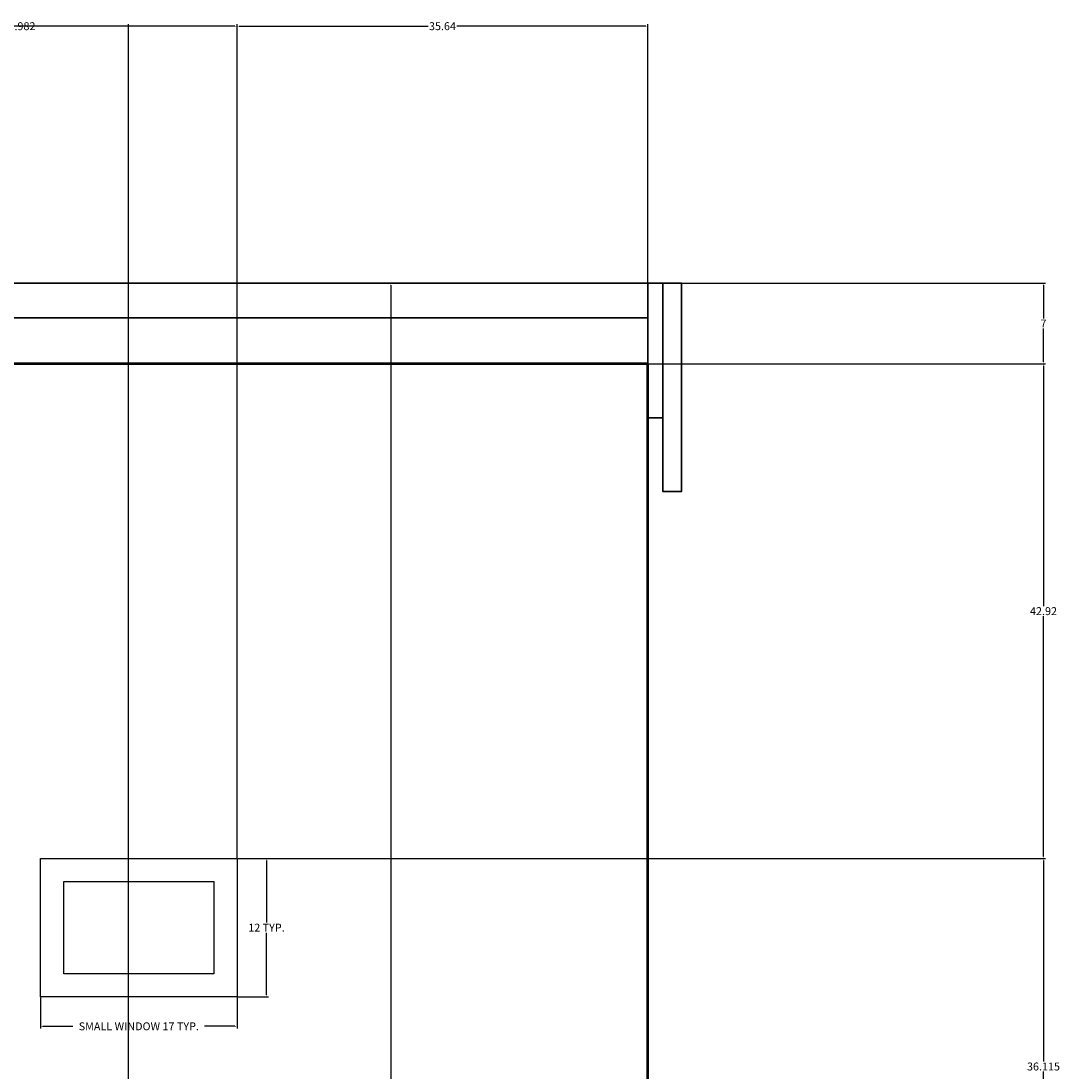
# Model space of a CAD drawing. Units: inches. Extents: x -139 to 346, y 72 to 413.
# Tile 18 of 18: x 256 to 346, y 322 to 413. Entities that reach past the tile are written whole.
import ezdxf

# ---------------------------------------------------------------- set-up
doc = ezdxf.new("R2010")
doc.units = ezdxf.units.IN
doc.header["$MEASUREMENT"] = 0
for name, color, linetype, lineweight in [('A-ANNO-DIMS', 2, 'Continuous', 18), ('A-GLAZ', 4, 'Continuous', 25), ('A-ROOF', 1, 'Continuous', 35), ('A-WALL', 7, 'Continuous', 50)]:
    doc.layers.add(name, color=color, linetype=linetype, lineweight=lineweight)
doc.styles.get("Standard").update_dxf_attribs({"font": 'arial.ttf'})
doc.dimstyles.get("Standard").update_dxf_attribs({"dimtxt": 0.6875, "dimasz": 0.18, "dimexe": 0.18, "dimexo": 0.0625, "dimgap": 0.09, "dimtad": 0, "dimtih": 1, "dimtoh": 1, "dimdec": 4, "dimzin": 0, "dimdsep": 46, "dimlunit": 4, "dimtxsty": 'Standard', "dimcen": 0.09, "dimadec": 0, "dimazin": 0, "dimtfac": 1, "dimtdec": 4, "dimtofl": 0, "dimtmove": 0, "dimatfit": 3, "dimfxl": 1, "dimtolj": 1, "dimtzin": 0, "dimarcsym": 0})

# ---------------------------------------------------------------- blocks, each defined once
blk = doc.blocks.new('WIN-SMALL')
for points in [[(0, 12.015), (17.035, 12.015), (17.035, 0), (0, 0)], [(2, 10.015), (15.035, 10.015), (15.035, 2), (2, 2)]]:
    blk.add_lwpolyline(points, close=True)
blk = doc.blocks.new('*D5')
at = {"layer": 'A-ANNO-DIMS', "color": 0, "lineweight": -2, "transparency": 16777216}
for p, q in [((257.212, 327.977), (257.212, 325.305)), ((274.247, 327.977), (274.247, 325.305)), ((257.392, 325.485), (260.019, 325.485)), ((274.067, 325.485), (271.439, 325.485))]:
    blk.add_line(p, q, dxfattribs=at)
at = {"layer": 'A-ANNO-DIMS', "color": 0, "transparency": 16777216}
for points in [[(257.392, 325.515), (257.392, 325.455), (257.212, 325.485)], [(274.067, 325.515), (274.067, 325.455), (274.247, 325.485)]]:
    blk.add_solid(points, dxfattribs=at)
at = {"layer": 'Defpoints', "color": 0, "transparency": 16777216}
for p in [(257.212, 328.04), (274.247, 328.04), (274.247, 325.485)]:
    blk.add_point(p, dxfattribs=at)
at = {"layer": 'A-ANNO-DIMS', "color": 0, "transparency": 16777216, "insert": (265.729, 325.485), "char_height": 0.6875, "attachment_point": 5}
blk.add_mtext('\\A1;SMALL WINDOW 17 TYP.', dxfattribs=at)
blk = doc.blocks.new('*D6')
at = {"layer": 'A-ANNO-DIMS', "color": 0, "lineweight": -2, "transparency": 16777216}
for p, q in [((274.309, 340.055), (276.982, 340.055)), ((276.802, 339.875), (276.802, 334.483)), ((276.802, 328.22), (276.802, 333.612)), ((274.309, 328.04), (276.982, 328.04))]:
    blk.add_line(p, q, dxfattribs=at)
at = {"layer": 'A-ANNO-DIMS', "color": 0, "transparency": 16777216}
for points in [[(276.772, 339.875), (276.832, 339.875), (276.802, 340.055)], [(276.772, 328.22), (276.832, 328.22), (276.802, 328.04)]]:
    blk.add_solid(points, dxfattribs=at)
at = {"layer": 'Defpoints', "color": 0, "transparency": 16777216}
for p in [(274.247, 340.055), (276.802, 340.055), (274.247, 328.04)]:
    blk.add_point(p, dxfattribs=at)
at = {"layer": 'A-ANNO-DIMS', "color": 0, "transparency": 16777216, "insert": (276.802, 334.047), "char_height": 0.6875, "attachment_point": 5}
blk.add_mtext('\\A1;12 TYP.', dxfattribs=at)
blk = doc.blocks.new('*D28')
at = {"layer": 'A-ANNO-DIMS', "color": 0, "lineweight": -2, "transparency": 16777216}
for p, q in [((175.668, 340.117), (175.668, 412.455)), ((175.848, 412.275), (223.706, 412.275)), ((274.067, 412.275), (226.208, 412.275)), ((274.247, 340.117), (274.247, 412.455))]:
    blk.add_line(p, q, dxfattribs=at)
at = {"layer": 'A-ANNO-DIMS', "color": 0, "transparency": 16777216}
for points in [[(175.848, 412.305), (175.848, 412.245), (175.668, 412.275)], [(274.067, 412.305), (274.067, 412.245), (274.247, 412.275)]]:
    blk.add_solid(points, dxfattribs=at)
at = {"layer": 'Defpoints', "color": 0, "transparency": 16777216}
for p in [(274.247, 412.275), (175.668, 340.055), (274.247, 340.055)]:
    blk.add_point(p, dxfattribs=at)
at = {"layer": 'A-ANNO-DIMS', "color": 0, "transparency": 16777216, "insert": (224.957, 412.275), "char_height": 0.6875, "attachment_point": 5}
blk.add_mtext('\\A1;98.58', dxfattribs=at)
blk = doc.blocks.new('*D29')
at = {"layer": 'A-ANNO-DIMS', "color": 0, "lineweight": -2, "transparency": 16777216}
for p, q in [((274.247, 340.117), (274.247, 412.455)), ((274.427, 412.275), (290.82, 412.275)), ((309.709, 412.275), (293.316, 412.275)), ((309.889, 383.037), (309.889, 412.455))]:
    blk.add_line(p, q, dxfattribs=at)
at = {"layer": 'A-ANNO-DIMS', "color": 0, "transparency": 16777216}
for points in [[(274.427, 412.305), (274.427, 412.245), (274.247, 412.275)], [(309.709, 412.305), (309.709, 412.245), (309.889, 412.275)]]:
    blk.add_solid(points, dxfattribs=at)
at = {"layer": 'Defpoints', "color": 0, "transparency": 16777216}
for p in [(309.889, 412.275), (309.889, 382.975), (274.247, 340.055)]:
    blk.add_point(p, dxfattribs=at)
at = {"layer": 'A-ANNO-DIMS', "color": 0, "transparency": 16777216, "insert": (292.068, 412.275), "char_height": 0.6875, "attachment_point": 5}
blk.add_mtext('\\A1;35.64', dxfattribs=at)
blk = doc.blocks.new('*D31')
at = {"layer": 'A-ANNO-DIMS', "color": 0, "lineweight": -2, "transparency": 16777216}
for p, q in [((309.827, 389.975), (287.409, 389.975)), ((287.589, 389.795), (287.589, 242.916)), ((287.589, 95.155), (287.589, 242.034)), ((309.827, 94.975), (287.409, 94.975))]:
    blk.add_line(p, q, dxfattribs=at)
at = {"layer": 'A-ANNO-DIMS', "color": 0, "transparency": 16777216}
for points in [[(287.559, 389.795), (287.619, 389.795), (287.589, 389.975)], [(287.559, 95.155), (287.619, 95.155), (287.589, 94.975)]]:
    blk.add_solid(points, dxfattribs=at)
at = {"layer": 'Defpoints', "color": 0, "transparency": 16777216}
for p in [(287.589, 389.975), (309.889, 389.975), (309.889, 94.975)]:
    blk.add_point(p, dxfattribs=at)
at = {"layer": 'A-ANNO-DIMS', "color": 0, "transparency": 16777216, "insert": (287.589, 242.475), "char_height": 0.6875, "attachment_point": 5}
blk.add_mtext('\\A1;295', dxfattribs=at)
blk = doc.blocks.new('*D35')
at = {"layer": 'A-ANNO-DIMS', "color": 0, "lineweight": -2, "transparency": 16777216}
for p, q in [((274.309, 340.055), (344.386, 340.055)), ((344.206, 339.875), (344.206, 322.439)), ((344.206, 304.12), (344.206, 321.556)), ((274.309, 303.94), (344.386, 303.94))]:
    blk.add_line(p, q, dxfattribs=at)
at = {"layer": 'A-ANNO-DIMS', "color": 0, "transparency": 16777216}
for points in [[(344.176, 339.875), (344.236, 339.875), (344.206, 340.055)], [(344.176, 304.12), (344.236, 304.12), (344.206, 303.94)]]:
    blk.add_solid(points, dxfattribs=at)
at = {"layer": 'Defpoints', "color": 0, "transparency": 16777216}
for p in [(274.247, 340.055), (344.206, 340.055), (274.247, 303.94)]:
    blk.add_point(p, dxfattribs=at)
at = {"layer": 'A-ANNO-DIMS', "color": 0, "transparency": 16777216, "insert": (344.206, 321.998), "char_height": 0.6875, "attachment_point": 5}
blk.add_mtext('\\A1;36.115', dxfattribs=at)
blk = doc.blocks.new('*D36')
at = {"layer": 'A-ANNO-DIMS', "color": 0, "lineweight": -2, "transparency": 16777216}
for p, q in [((309.952, 382.975), (344.386, 382.975)), ((344.206, 382.795), (344.206, 361.956)), ((344.206, 340.235), (344.206, 361.074)), ((274.309, 340.055), (344.386, 340.055))]:
    blk.add_line(p, q, dxfattribs=at)
at = {"layer": 'A-ANNO-DIMS', "color": 0, "transparency": 16777216}
for points in [[(344.176, 382.795), (344.236, 382.795), (344.206, 382.975)], [(344.176, 340.235), (344.236, 340.235), (344.206, 340.055)]]:
    blk.add_solid(points, dxfattribs=at)
at = {"layer": 'Defpoints', "color": 0, "transparency": 16777216}
for p in [(309.889, 382.975), (344.206, 382.975), (274.247, 340.055)]:
    blk.add_point(p, dxfattribs=at)
at = {"layer": 'A-ANNO-DIMS', "color": 0, "transparency": 16777216, "insert": (344.206, 361.515), "char_height": 0.6875, "attachment_point": 5}
blk.add_mtext('\\A1;42.92', dxfattribs=at)
blk = doc.blocks.new('*D37')
at = {"layer": 'A-ANNO-DIMS', "color": 0, "lineweight": -2, "transparency": 16777216}
for p, q in [((309.951928, 389.974785), (344.385522, 389.974785)), ((344.205522, 389.794785), (344.205522, 386.908535)), ((344.205522, 383.154785), (344.205522, 386.041035)), ((309.951928, 382.974785), (344.385522, 382.974785))]:
    blk.add_line(p, q, dxfattribs=at)
at = {"layer": 'A-ANNO-DIMS', "color": 0, "transparency": 16777216}
for points in [[(344.175522, 389.794785), (344.235522, 389.794785), (344.205522, 389.974785)], [(344.175522, 383.154785), (344.235522, 383.154785), (344.205522, 382.974785)]]:
    blk.add_solid(points, dxfattribs=at)
at = {"layer": 'Defpoints', "color": 0, "transparency": 16777216}
for p in [(309.889428, 389.974785), (344.205522, 389.974785), (309.889428, 382.974785)]:
    blk.add_point(p, dxfattribs=at)
at = {"layer": 'A-ANNO-DIMS', "color": 0, "transparency": 16777216, "insert": (344.205522, 386.474785), "char_height": 0.6875, "attachment_point": 5}
blk.add_mtext('\\A1;7', dxfattribs=at)
blk = doc.blocks.new('*D82')
at = {"layer": 'A-ANNO-DIMS', "color": 0, "lineweight": -2, "transparency": 16777216}
for p, q in [((245.84, 184.668), (245.84, 412.455)), ((246.02, 412.275), (253.85, 412.275)), ((264.642, 412.275), (256.812, 412.275)), ((264.822, 184.668), (264.822, 412.455))]:
    blk.add_line(p, q, dxfattribs=at)
at = {"layer": 'A-ANNO-DIMS', "color": 0, "transparency": 16777216}
for points in [[(246.02, 412.305), (246.02, 412.245), (245.84, 412.275)], [(264.642, 412.305), (264.642, 412.245), (264.822, 412.275)]]:
    blk.add_solid(points, dxfattribs=at)
at = {"layer": 'Defpoints', "color": 0, "transparency": 16777216}
for p in [(264.822, 412.275), (245.84, 184.606), (264.822, 184.606)]:
    blk.add_point(p, dxfattribs=at)
at = {"layer": 'A-ANNO-DIMS', "color": 0, "transparency": 16777216, "insert": (255.331, 412.275), "char_height": 0.6875, "attachment_point": 5}
blk.add_mtext('\\A1;18.982', dxfattribs=at)

msp = doc.modelspace()

# ---------------------------------------------------------------- linework, layer by layer
at = {"layer": 'A-ROOF'}
for p, q in [((-47.2734, 389.9748), (309.8894, 389.9748)), ((309.8894, 389.9748), (309.8894, 386.9223)), ((-47.2734, 386.9748), (309.8894, 386.9748)), ((309.8894, 386.9748), (309.8894, 382.9748))]:
    msp.add_line(p, q, dxfattribs=at)
for points in [[(309.8894, 389.9748), (311.1776, 389.9748), (311.1776, 378.2896), (309.8894, 378.2896)], [(311.1776, 389.9748), (312.8172, 389.9748), (312.8172, 371.9089), (311.1776, 371.9089)]]:
    msp.add_lwpolyline(points, close=True, dxfattribs=at)
at = {"layer": 'A-WALL'}
for p, q in [((309.8894, 382.9748), (89.4597, 382.9748)), ((309.8894, 94.9748), (309.8894, 382.9748))]:
    msp.add_line(p, q, dxfattribs=at)

# ---------------------------------------------------------------- block references
at = {"layer": 'A-GLAZ'}
msp.add_blockref('WIN-SMALL', (257.212, 328.04), dxfattribs=at)

# ---------------------------------------------------------------- dimensions: what is measured, and where the dimension line sits
at = {"layer": 'A-ANNO-DIMS'}
for base, p1, p2, override, picture, middle in [((274.2465, 412.2748), (175.6676, 340.0548), (274.2465, 340.0548), {"dimdec": 2, "dimlfac": 1, "dimrnd": 0, "dimzin": 0, "dimdsep": 46, "dimlunit": 2}, '*D28', (224.957, 412.2748)), ((264.8219, 412.2748), (245.8399, 184.6055), (264.8219, 184.6055), {"dimdec": 3, "dimlfac": 1, "dimrnd": 0, "dimzin": 0, "dimdsep": 46, "dimlunit": 2}, '*D82', (255.3309, 412.2748)), ((309.8894, 412.2748), (274.2465, 340.0548), (309.8894, 382.9748), {"dimdec": 2, "dimlfac": 1, "dimrnd": 0, "dimzin": 0, "dimdsep": 46, "dimlunit": 2}, '*D29', (292.068, 412.2748))]:
    dim = msp.add_linear_dim(base=base, p1=p1, p2=p2, dimstyle='Standard', override=override, dxfattribs=at)
    dim.commit()
    dim.dimension.update_dxf_attribs({"geometry": picture, "text_midpoint": middle})
for base, p1, p2, override, picture, middle in [((287.5894, 389.9748), (309.8894, 94.9748), (309.8894, 389.9748), {"dimdec": 0, "dimlfac": 1, "dimrnd": 0, "dimzin": 0, "dimdsep": 46, "dimlunit": 2}, '*D31', (287.5894, 242.4748)), ((344.2055, 389.9748), (309.8894, 382.9748), (309.8894, 389.9748), {"dimdec": 0, "dimlfac": 1, "dimrnd": 0, "dimzin": 0, "dimdsep": 46, "dimlunit": 2}, '*D37', (344.2055, 386.4748)), ((344.2055, 382.9748), (274.2465, 340.0548), (309.8894, 382.9748), {"dimdec": 2, "dimlfac": 1, "dimrnd": 0, "dimzin": 0, "dimdsep": 46, "dimlunit": 2}, '*D36', (344.2055, 361.5148)), ((344.2055, 340.0548), (274.2465, 303.9402), (274.2465, 340.0548), {"dimdec": 3, "dimlfac": 1, "dimrnd": 0, "dimzin": 0, "dimdsep": 46, "dimlunit": 2}, '*D35', (344.2055, 321.9975))]:
    dim = msp.add_linear_dim(base=base, p1=p1, p2=p2, angle=90, dimstyle='Standard', override=override, dxfattribs=at)
    dim.commit()
    dim.dimension.update_dxf_attribs({"geometry": picture, "text_midpoint": middle})
dim = msp.add_linear_dim(base=(276.8018, 340.0548), p1=(274.2465, 328.0398), p2=(274.2465, 340.0548), angle=90, text='<> TYP.', dimstyle='Standard', override={"dimdec": 0, "dimlfac": 1, "dimrnd": 0, "dimzin": 0, "dimdsep": 46, "dimlunit": 2}, dxfattribs=at)
dim.commit()
dim.dimension.update_dxf_attribs({"geometry": '*D6', "text_midpoint": (276.8018, 334.0473)})
dim = msp.add_linear_dim(base=(274.2465, 325.4846), p1=(257.2116, 328.0398), p2=(274.2465, 328.0398), text='SMALL WINDOW <> TYP.', dimstyle='Standard', override={"dimdec": 0, "dimlfac": 1, "dimrnd": 0, "dimzin": 0, "dimdsep": 46, "dimlunit": 2}, dxfattribs=at)
dim.commit()
dim.dimension.update_dxf_attribs({"geometry": '*D5', "text_midpoint": (265.7291, 325.4846)})

doc.saveas('drawing.dxf')
